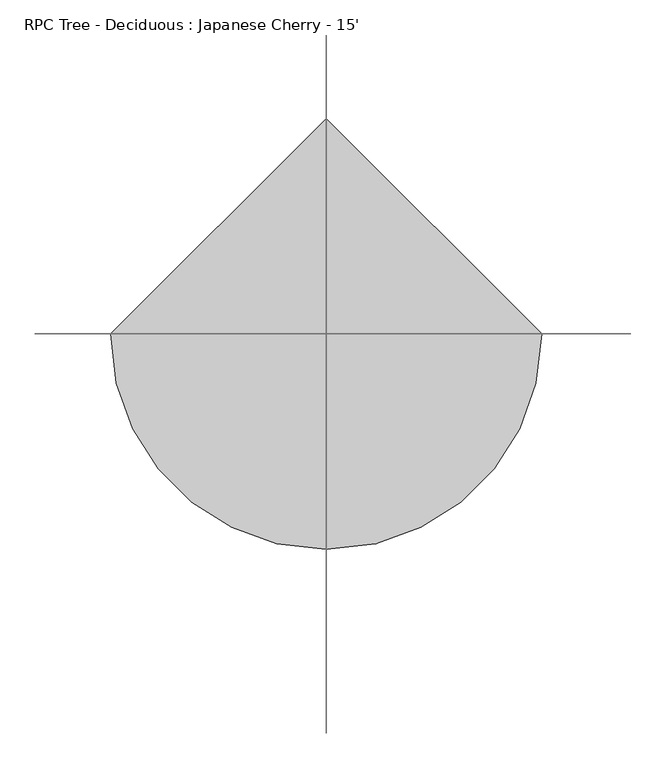
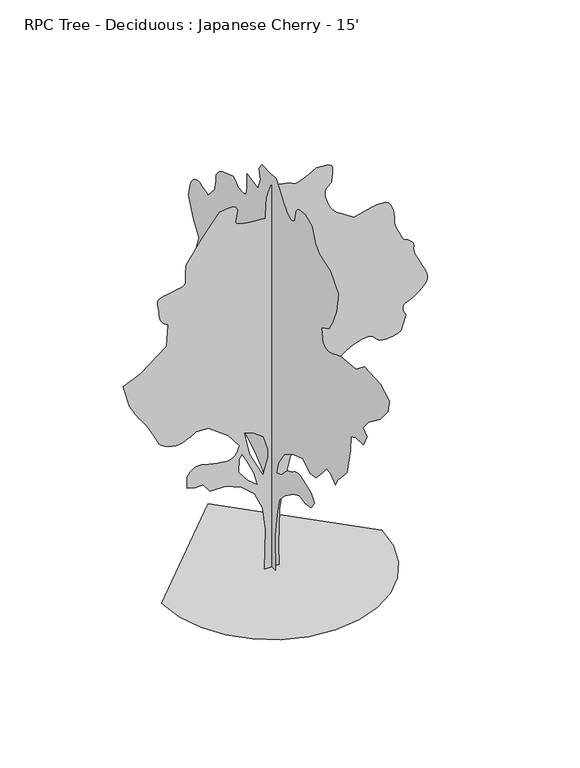
"""IFC4 building model written with IfcOpenShell, lengths in millimetres: geographic element geometry, RPC Tree - Deciduous : Japanese Cherry - 15'."""

from ifc_helpers import new_model, si_unit, origin, place, context, project, spatial, triangles, source, transform, mapped, element, save


def rpc_tree_deciduous_japanese_cherry_15_720dba75(model_context):
    return source(origin(), model_context, "Body", "Tessellation", [
        triangles([(-0.001308, 35.3573372, 0.0027784), (-0.001308, -34.1823135, 0.0027784), (-0.001308, -27.86057, 186.4945759), (-0.001308, -46.8258028, 309.7693188), (-0.001308, -68.9520821, 404.5960888), (-0.001308, -119.526734, 458.3308539), (-0.001308, -195.3869473, 512.0667818), (-0.001308, -245.9616038, 534.1922482), (-0.001308, -296.5362602, 524.7095421), (-0.001308, -350.2710254, 534.1922482), (-0.001308, -378.7190346, 575.2842167), (-0.001308, -350.2710254, 613.2148956), (-0.001308, -249.1228934, 647.984285), (-0.001308, -240.3312607, 647.275462), (-0.001308, -231.6226171, 646.3722467), (-0.001308, -223.0799154, 645.0814098), (-0.001308, -214.7861266, 643.2109571), (-0.001308, -206.8242398, 640.5664965), (-0.001308, -199.2760268, 636.9536356), (-0.001308, -192.2268386, 632.1802351), (-0.001308, -185.1764696, 627.0382524), (-0.001308, -177.6294557, 622.3929691), (-0.001308, -169.6675688, 618.1636488), (-0.001308, -161.37378, 614.2651222), (-0.001308, -152.8310783, 610.6166531), (-0.001308, -144.1224257, 607.1329631), (-0.001308, -135.3308021, 603.7322259), (-0.001308, -87.917308, 553.1575876), (-0.001308, -40.5040593, 534.1922482), (-0.001308, -59.4694078, 600.5709363), (-0.001308, -113.2044001, 679.5936201), (-0.001308, -189.0655672, 727.0070051), (-0.001308, -277.5709208, 755.4550507), (-0.001308, -340.7883556, 714.3630095), (-0.001308, -391.3629939, 720.6855886), (-0.001308, -445.0977591, 777.5804443), (-0.001308, -486.1897639, 828.1551189), (-0.001308, -524.1192438, 824.9938293), (-0.001308, -565.2112487, 787.0643131), (-0.001308, -590.4979683, 831.3164085), (-0.001308, -618.9460138, 862.9245083), (-0.001308, -669.5206884, 916.6604725), (-0.001308, -701.1287882, 1058.9006275), (-0.001308, -704.2900778, 1134.7619854), (-0.001308, -748.5433359, 1153.7261621), (-0.001308, -818.0821873, 1160.0487413), (-0.001308, -846.5301601, 1220.1000904), (-0.001308, -811.7607708, 1248.5482086), (-0.001308, -859.1741558, 1305.4441544), (-0.001308, -966.6436861, 1387.6352131), (-0.001308, -1036.1837002, 1469.8144993), (-0.001308, -1048.8264605, 1536.1932964), (-0.001308, -969.8049757, 1580.4417583), (-0.001308, -824.4035311, 1586.7714592), (-0.001308, -751.7034628, 1529.8753681), (-0.001308, -612.6245974, 1514.0631065), (-0.001308, -593.7327636, 1506.6546925), (-0.001308, -575.2842167, 1499.4952457), (-0.001308, -557.7187554, 1492.8337337), (-0.001308, -541.4820285, 1486.9188332), (-0.001308, -527.0138346, 1481.999802), (-0.001308, -514.7574969, 1478.3251717), (-0.001308, -505.1539043, 1476.1322823), (-0.001308, -496.556682, 1476.0138302), (-0.001308, -487.4604349, 1477.886681), (-0.001308, -478.5312924, 1481.0277683), (-0.001308, -470.4307331, 1484.7259438), (-0.001308, -463.8236873, 1488.2582863), (-0.001308, -459.3727598, 1490.9015842), (-0.001308, -457.7405557, 1491.9446892), (-0.001308, -441.9364695, 1567.8060471), (-0.001308, -508.3151939, 1602.5719482), (-0.001308, -539.9244927, 1653.150111), (-0.001308, -574.6939184, 1735.3293972), (-0.001308, -593.6592579, 1839.6388733), (-0.001308, -520.9591533, 1921.8180141), (-0.001308, -426.1324196, 1956.5956879), (-0.001308, -388.2017043, 1991.3615891), (-0.001308, -359.7536951, 2067.2229469), (-0.001308, -293.3749706, 2092.506142), (-0.001308, -282.5647293, 2092.4587612), (-0.001308, -271.9216108, 2092.1387226), (-0.001308, -261.6091952, 2091.2615959), (-0.001308, -251.7946416, 2089.5664959), (-0.001308, -242.6438557, 2086.7454472), (-0.001308, -234.3228157, 2082.5612549), (-0.001308, -226.9962643, 2076.705653), (-0.001308, -221.0518052, 2069.380228), (-0.001308, -216.6008778, 2061.0592243), (-0.001308, -213.3945509, 2051.9084747), (-0.001308, -211.1827128, 2042.0939575), (-0.001308, -209.7176315, 2031.7815056), (-0.001308, -208.7492131, 2021.1372425), (-0.001308, -208.0309067, 2010.3270012), (-0.001308, -202.5760071, 2004.3054211), (-0.001308, -196.8982468, 1998.7580853), (-0.001308, -190.7795614, 1994.1589474), (-0.001308, -183.9970721, 1990.9585613), (-0.001308, -176.3303344, 1989.6427986), (-0.001308, -167.5564877, 1990.674131), (-0.001308, -157.4562502, 1994.5263668), (-0.001308, -147.4484763, 2000.1212288), (-0.001308, -138.9342158, 2006.0596745), (-0.001308, -131.6633751, 2012.2709232), (-0.001308, -125.3870322, 2018.7073036), (-0.001308, -119.857446, 2025.2977444), (-0.001308, -114.8262942, 2032.0066372), (-0.001308, -110.0434738, 2038.7749741), (-0.001308, -65.7911513, 2098.8358429), (-0.001308, -37.3431262, 2133.6017441), (-0.001308, 10.0702679, 2130.436821), (-0.001308, 85.931519, 2133.6017441), (-0.001308, 114.3794283, 2095.6710651), (-0.001308, 101.7359413, 2041.9397518), (-0.001308, 123.8626885, 1981.878883), (-0.001308, 221.8495399, 2000.8442951), (-0.001308, 221.8495399, 1931.3007202), (-0.001308, 222.5773298, 1920.5378597), (-0.001308, 223.6097523, 1910.1424187), (-0.001308, 225.250259, 1900.529488), (-0.001308, 227.8034643, 1892.0898869), (-0.001308, 231.5716391, 1885.1794075), (-0.001308, 236.8617959, 1880.2128502), (-0.001308, 243.976169, 1877.5695522), (-0.001308, 252.1040159, 1876.585746), (-0.001308, 260.2318447, 1876.2655621), (-0.001308, 268.3596734, 1876.490839), (-0.001308, 276.4875203, 1877.1665245), (-0.001308, 284.6153491, 1878.1740211), (-0.001308, 292.7443769, 1879.3948769), (-0.001308, 300.8722238, 1880.73433), (-0.001308, 308.3267833, 1888.1071358), (-0.001308, 315.8097931, 1895.0769138), (-0.001308, 323.3485408, 1901.216946), (-0.001308, 330.9690422, 1906.1122868), (-0.001308, 338.700983, 1909.3482811), (-0.001308, 346.5715782, 1910.5099834), (-0.001308, 354.6069889, 1909.1823029), (-0.001308, 439.9510529, 1880.73433), (-0.001308, 452.0604155, 1872.5793045), (-0.001308, 463.6719523, 1864.2581554), (-0.001308, 474.2878015, 1855.6051952), (-0.001308, 483.4113361, 1846.4544456), (-0.001308, 490.5434953, 1836.6399284), (-0.001308, 495.1876159, 1825.9956654), (-0.001308, 496.8470713, 1814.3556782), (-0.001308, 497.2157261, 1802.4311153), (-0.001308, 498.2481485, 1791.0164051), (-0.001308, 499.8329355, 1780.0164951), (-0.001308, 501.859883, 1769.3485416), (-0.001308, 504.218678, 1758.9174923), (-0.001308, 506.7991528, 1748.6643391), (-0.001308, 509.4898679, 1738.494175), (-0.001308, 569.5472122, 1672.1155231), (-0.001308, 587.8120131, 1680.1164883), (-0.001308, 605.9393223, 1687.4063049), (-0.001308, 623.7892502, 1693.2619068), (-0.001308, 641.2243778, 1696.9600822), (-0.001308, 658.1070683, 1697.7780556), (-0.001308, 674.2987398, 1695.0043877), (-0.001308, 689.6606655, 1687.9160122), (-0.001308, 702.99568, 1676.963483), (-0.001308, 713.5108086, 1663.3439655), (-0.001308, 721.6753538, 1647.5197861), (-0.001308, 727.9599993, 1629.9294353), (-0.001308, 732.8352831, 1611.0115494), (-0.001308, 736.7705807, 1591.2046188), (-0.001308, 740.2353401, 1570.9590523), (-0.001308, 699.1433716, 1463.4967163), (-0.001308, 648.5698597, 1393.9531414), (-0.001308, 689.6606655, 1280.1609592), (-0.001308, 651.7299866, 1220.1000904), (-0.001308, 636.2483007, 1214.6475889), (-0.001308, 621.3474661, 1208.9698832), (-0.001308, 607.6070984, 1202.8535414), (-0.001308, 595.6079398, 1196.073432), (-0.001308, 585.9320769, 1188.404278), (-0.001308, 579.1590892, 1179.6316303), (-0.001308, 575.8685924, 1169.5313747), (-0.001308, 574.7911145, 1158.7863184), (-0.001308, 574.2102997, 1148.2060776), (-0.001308, 574.0443578, 1137.7656538), (-0.001308, 574.2102997, 1127.4354704), (-0.001308, 574.6251726, 1117.1870407), (-0.001308, 575.2059875, 1106.9955116), (-0.001308, 575.8685924, 1096.8301437), (-0.001308, 563.2257957, 1046.2566319), (-0.001308, 474.7204422, 1055.7393379), (-0.001308, 467.3666396, 1040.9024529), (-0.001308, 460.5936519, 1026.4520994), (-0.001308, 454.9810947, 1012.776844), (-0.001308, 451.1109821, 1000.2621283), (-0.001308, 449.5629298, 989.2965912), (-0.001308, 450.9177526, 980.2643663), (-0.001308, 455.7551027, 973.5565636), (-0.001308, 463.5972839, 967.9901882), (-0.001308, 473.2091609, 962.3136452), (-0.001308, 484.03717, 956.8030077), (-0.001308, 495.5289831, 951.7344944), (-0.001308, 507.1310366, 947.3843239), (-0.001308, 518.2909658, 944.0298775), (-0.001308, 528.4552073, 941.9472284), (-0.001308, 537.6616948, 940.1312782), (-0.001308, 546.3703566, 937.4868176), (-0.001308, 554.6641454, 934.1512653), (-0.001308, 562.626014, 930.2621859), (-0.001308, 570.3401871, 925.9582335), (-0.001308, 577.8872191, 921.3781351), (-0.001308, 585.3512621, 916.6604725), (-0.001308, 658.0525658, 954.5911514), (-0.001308, 678.9523802, 959.9263636), (-0.001308, 699.2725788, 964.7648764), (-0.001308, 718.4310751, 968.6077377), (-0.001308, 735.8483986, 970.9570856), (-0.001308, 750.9436255, 971.3162207), (-0.001308, 763.1359772, 969.1885889), (-0.001308, 771.8434399, 964.0738575), (-0.001308, 777.6042074, 956.6548336), (-0.001308, 781.5382696, 948.0754154), (-0.001308, 783.9528025, 938.5286871), (-0.001308, 785.1512032, 928.2068607), (-0.001308, 785.4368689, 917.3052732), (-0.001308, 785.1144321, 906.0162094), (-0.001308, 784.4874355, 894.5338434), (-0.001308, 773.6226191, 883.1154997), (-0.001308, 762.591897, 872.2791698), (-0.001308, 751.2292912, 862.6021442), (-0.001308, 739.3688232, 854.6675268), (-0.001308, 726.8445877, 849.0560961), (-0.001308, 713.4918417, 846.3464504), (-0.001308, 699.1433716, 847.1204584), (-0.001308, 683.9473515, 850.4560106), (-0.001308, 668.5296879, 854.4564932), (-0.001308, 653.4439808, 858.2341696), (-0.001308, 639.2436848, 860.9071169), (-0.001308, 626.4800016, 861.5886887), (-0.001308, 615.7076941, 859.3957993), (-0.001308, 607.4778912, 853.4418749), (-0.001308, 601.257268, 845.775119), (-0.001308, 596.0322962, 838.9369463), (-0.001308, 591.6359076, 832.7909552), (-0.001308, 587.9044856, 827.1974012), (-0.001308, 584.6696903, 822.0174849), (-0.001308, 581.7668152, 817.1149498), (-0.001308, 579.029882, 812.3510691), (-0.001308, 589.8021895, 810.9227406), (-0.001308, 600.1880745, 809.0522879), (-0.001308, 609.7999878, 806.2963514), (-0.001308, 618.2501987, 802.2141151), (-0.001308, 625.1523937, 796.3620741), (-0.001308, 630.1201138, 788.2982494), (-0.001308, 632.7646471, 777.5804443), (-0.001308, 633.8432877, 765.0206732), (-0.001308, 634.4240662, 751.795899), (-0.001308, 634.5900444, 738.0187603), (-0.001308, 634.4240662, 723.7994974), (-0.001308, 634.0092659, 709.2483507), (-0.001308, 633.4284147, 694.4767233), (-0.001308, 632.7646471, 679.5936201), (-0.001308, 616.5279202, 667.4937046), (-0.001308, 600.4002708, 655.9462263), (-0.001308, 584.494265, 645.5058025), (-0.001308, 568.9201429, 636.7236351), (-0.001308, 553.7893441, 630.1533239), (-0.001308, 539.2097471, 626.3472336), (-0.001308, 525.2951168, 625.8588913), (-0.001308, 511.3792874, 627.5811699), (-0.001308, 496.8008532, 629.9684515), (-0.001308, 481.6688916, 632.908025), (-0.001308, 466.0947696, 636.2897953), (-0.001308, 450.1887637, 640.0046848), (-0.001308, 434.0623135, 643.938747), (-0.001308, 417.8244238, 647.984285), (-0.001308, 322.9976538, 625.8588913), (-0.001308, 212.366852, 568.9628366), (-0.001308, 149.1494262, 534.1922482), (-0.001308, 76.4488493, 474.1360665), (-0.001308, 32.1964064, 382.4706224), (-0.001308, 19.5529194, 252.8732822), (-0.001308, 32.1964064, 123.2771319), (37.4314339, 0.0001191, 0.0), (-38.42984, 0.0001191, 0.0), (-32.1080988, 0.0001042, 214.9402233), (-47.9123962, 9.43e-05, 338.2150025), (-89.0040241, 8.93e-05, 426.719157), (-155.3831028, 8.93e-05, 486.7765014), (-237.5658772, 8.43e-05, 521.5458907), (-316.5873619, 8.43e-05, 521.5458907), (-354.5192762, 8.43e-05, 568.9592757), (-395.6100457, 8.43e-05, 568.9592757), (-436.7020506, 8.43e-05, 578.4419455), (-436.7020506, 7.94e-05, 638.4992535), (-428.5185021, 7.94e-05, 649.2348627), (-420.0030699, 7.94e-05, 659.3623695), (-410.8249964, 7.44e-05, 668.2736715), (-400.6512714, 7.44e-05, 675.3608116), (-389.1499749, 7.44e-05, 680.014452), (-375.9904221, 7.44e-05, 681.6276529), (-360.8406564, 7.44e-05, 679.5912947), (-342.8520015, 7.44e-05, 675.0383749), (-322.2094025, 7.44e-05, 669.8774254), (-300.1290097, 7.94e-05, 664.6619734), (-277.8281362, 7.94e-05, 659.943148), (-256.5217514, 7.94e-05, 656.275712), (-237.4272047, 7.94e-05, 654.2108671), (-221.7606282, 7.94e-05, 654.3033033), (-209.3205445, 7.94e-05, 657.1327091), (-198.8706373, 7.94e-05, 662.6160954), (-190.0790228, 7.44e-05, 670.3112652), (-182.6137808, 7.44e-05, 679.7750044), (-176.1454074, 7.44e-05, 690.5662788), (-170.3396572, 7.44e-05, 702.2418016), (-164.8657725, 7.44e-05, 714.360684), (-221.7606282, 6.95e-05, 790.2220419), (-326.070068, 6.45e-05, 866.0834724), (-389.2886656, 6.45e-05, 869.2435266), (-399.4896418, 6.45e-05, 863.1616304), (-409.939549, 6.45e-05, 857.1626507), (-420.8884809, 6.45e-05, 851.3295765), (-432.5818079, 6.45e-05, 845.7443069), (-445.2720217, 6.45e-05, 840.4920839), (-459.2056189, 6.45e-05, 835.6535711), (-474.6327295, 6.95e-05, 831.3128477), (-492.3807378, 6.95e-05, 829.8110498), (-512.1201216, 6.95e-05, 832.8431322), (-532.3573311, 6.45e-05, 839.5236837), (-551.6000519, 6.45e-05, 848.9696188), (-568.3535714, 6.45e-05, 860.2954536), (-581.1255389, 6.45e-05, 872.6170126), (-588.42364, 6.45e-05, 885.0488119), (-594.7924373, 6.45e-05, 900.5482292), (-604.9199441, 5.95e-05, 921.1908646), (-617.5354895, 5.95e-05, 944.764789), (-631.3682934, 5.95e-05, 969.0558208), (-645.1454321, 5.95e-05, 991.8545019), (-657.5950356, 5.46e-05, 1010.9491213), (-667.4463238, 5.46e-05, 1024.1276047), (-675.7590431, 5.46e-05, 1034.6237663), (-684.4025562, 5.46e-05, 1046.9453253), (-693.323378, 5.46e-05, 1060.7864862), (-702.4646805, 5.46e-05, 1075.8437794), (-711.7718885, 4.96e-05, 1091.8149702), (-721.1905724, 4.96e-05, 1108.3930281), (-730.6637587, 4.96e-05, 1125.2757912), (-765.4343834, 4.47e-05, 1245.3952034), (-673.7677402, 3.97e-05, 1283.3258823), (-541.011454, 3.47e-05, 1387.6352131), (-534.6888748, 2.48e-05, 1501.4154774), (-544.1075586, 2.48e-05, 1508.2548855), (-553.1386208, 2.48e-05, 1515.4143322), (-561.3956386, 2.48e-05, 1523.2375465), (-568.491063, 2.48e-05, 1532.0563396), (-574.0384352, 2.48e-05, 1542.2028133), (-577.6513324, 2.48e-05, 1554.0087788), (-578.9421693, 2.48e-05, 1567.7942745), (-580.0848321, 1.98e-05, 1583.3221058), (-582.6641078, 1.98e-05, 1599.51385), (-585.4105245, 1.98e-05, 1615.4920898), (-587.051013, 1.98e-05, 1630.3561535), (-586.3137397, 1.98e-05, 1643.2289143), (-581.9268345, 1.98e-05, 1653.2213276), (-572.6195901, 1.98e-05, 1659.4680393), (-556.3176782, 1.98e-05, 1663.3914917), (-533.9338337, 1.49e-05, 1667.2675632), (-508.6743653, 1.49e-05, 1671.4043747), (-483.7467808, 1.49e-05, 1676.1693455), (-462.357425, 1.49e-05, 1681.8589691), (-447.7138058, 1.49e-05, 1688.8287472), (-443.0234307, 1.49e-05, 1697.3987183), (-444.0096351, 1.49e-05, 1707.7111702), (-444.3320354, 1.49e-05, 1719.5169903), (-444.1009086, 1.49e-05, 1732.5675018), (-443.4288202, 1.49e-05, 1746.601965), (-442.4248481, 9.9e-06, 1761.3949574), (-441.1991961, 9.9e-06, 1776.6857391), (-439.8621411, 9.9e-06, 1792.2254883), (-360.8406564, 5e-06, 1906.0175251), (-269.1751941, -5e-06, 2019.8095619), (-249.6657745, -5e-06, 2023.0574741), (-230.9588313, -5e-06, 2025.5111034), (-213.8544611, -5e-06, 2026.3645397), (-199.156303, -5e-06, 2024.7998096), (-187.6644899, -5e-06, 2020.0348389), (-180.1814801, -5e-06, 2011.2634266), (-177.508551, 0.0, 1997.679372), (-178.8266391, 0.0, 1982.3768177), (-181.8587215, 0.0, 1968.8876701), (-185.2227058, 0.0, 1957.1290855), (-187.5353009, 0.0, 1946.9589214), (-187.4155771, 0.0, 1938.2822708), (-183.4802613, 0.0, 1930.9924541), (-174.3484423, 0.0, 1924.9829372), (-160.497816, 0.0, 1920.1111416), (-143.6601447, 0.0, 1916.2469879), (-124.3356429, 5e-06, 1913.2006622), (-103.0207194, 5e-06, 1910.830022), (-80.2125185, 5e-06, 1908.9452534), (-56.4091114, 5e-06, 1907.3924412), (-32.1080988, 5e-06, 1906.0175251), (-28.9470476, 0.0, 1991.3615891), (-28.2097697, -5e-06, 2003.4639027), (-26.1455108, -5e-06, 2015.3883202), (-22.9754531, -5e-06, 2027.1823677), (-18.9206611, -5e-06, 2038.8697357), (-14.2023194, -5e-06, 2050.4742599), (-9.0417537, -5e-06, 2062.0193401), (-3.6599567, -5e-06, 2073.5408752), (17.9133643, -5e-06, 2069.4632172), (38.8784908, -5e-06, 2065.3383236), (58.6271082, -5e-06, 2061.1066051), (76.5511414, -5e-06, 2056.6972813), (92.0422743, -5e-06, 2052.074453), (104.4923138, -5e-06, 2047.1671944), (113.2929485, -5e-06, 2041.9279793), (124.7481359, -5e-06, 2040.3988575), (143.389885, -5e-06, 2045.1757462), (165.9586564, -5e-06, 2054.0420654), (189.1912136, -5e-06, 2064.793008), (209.824311, -5e-06, 2075.2002216), (224.5959566, -9.9e-06, 2083.0709621), (230.2452666, -9.9e-06, 2086.1883591), (234.7981318, -9.9e-06, 2086.2831207), (246.5388578, -9.9e-06, 2086.1527508), (262.5918387, -9.9e-06, 2085.192635), (280.0826315, -9.9e-06, 2082.7983044), (296.1356124, -5e-06, 2078.3532269), (307.8763384, -5e-06, 2071.2530788), (312.4292218, -5e-06, 2060.8932461), (312.244313, -5e-06, 2048.8858395), (311.7286832, -5e-06, 2037.2103893), (310.9357083, -5e-06, 2025.8192242), (309.9222528, -5e-06, 2014.6415634), (308.7428189, -5e-06, 2003.6297356), (307.4520184, 0.0, 1992.7247326), (306.1066426, 0.0, 1981.878883), (298.0523014, 0.0, 1975.7151604), (290.4412652, 0.0, 1969.2077087), (283.7133147, 0.0, 1961.9652729), (278.3129358, 0.0, 1953.6560417), (274.6822526, 0.0, 1943.9125957), (273.2634075, 0.0, 1932.3675156), (274.4985247, 0.0, 1918.6532364), (277.9442991, 5e-06, 1903.4572163), (282.717627, 5e-06, 1887.9767658), (288.598082, 5e-06, 1872.7096745), (295.3616045, 5e-06, 1858.1656494), (302.7888946, 5e-06, 1844.8424801), (310.6595261, 5e-06, 1833.2261833), (318.750602, 9.9e-06, 1823.8264664), (328.2605593, 9.9e-06, 1815.2445774), (340.2596815, 9.9e-06, 1805.82117), (354.3308066, 9.9e-06, 1795.7103046), (370.0625499, 9.9e-06, 1785.0541237), (387.0365501, 9.9e-06, 1773.9712246), (404.8402599, 9.9e-06, 1762.6275856), (423.0600417, 9.9e-06, 1751.1298862), (454.760614, 9.9e-06, 1759.8065369), (485.6598907, 9.9e-06, 1767.677132), (514.95545, 9.9e-06, 1773.9357616), (541.8471225, 9.9e-06, 1777.7999153), (565.5300882, 9.9e-06, 1778.4519104), (585.2054498, 9.9e-06, 1775.0973186), (600.0695498, 9.9e-06, 1766.9303753), (610.7778351, 9.9e-06, 1753.6545868), (618.7764748, 1.49e-05, 1736.5621708), (624.4530905, 1.49e-05, 1717.2530296), (628.1951586, 1.49e-05, 1697.3394196), (630.388048, 1.49e-05, 1678.4215336), (631.4204704, 1.98e-05, 1662.0994194), (631.6788849, 1.98e-05, 1649.9853333), (634.1301161, 1.98e-05, 1637.0651917), (640.4515326, 1.98e-05, 1619.000742), (649.094973, 1.98e-05, 1598.3995285), (658.5136568, 2.48e-05, 1577.8458412), (667.15826, 2.48e-05, 1559.9473698), (673.4796764, 2.48e-05, 1547.2997406), (675.9309803, 2.48e-05, 1542.5110794), (679.2392086, 2.48e-05, 1541.1953167), (687.6894922, 2.48e-05, 1537.3904617), (699.0710649, 2.48e-05, 1531.3215008), (711.1709078, 2.48e-05, 1523.2019382), (721.7773098, 2.48e-05, 1513.2570511), (728.6795048, 2.48e-05, 1501.7118256), (729.6657091, 2.98e-05, 1488.7799114), (728.4306101, 2.98e-05, 1475.5515038), (729.8506542, 2.98e-05, 1462.7143513), (733.4813192, 2.98e-05, 1449.8771988), (738.8817163, 2.98e-05, 1436.660709), (745.608486, 2.98e-05, 1422.6618542), (753.2206667, 3.47e-05, 1407.5014423), (761.2750443, 3.47e-05, 1390.7882183), (770.4720119, 3.47e-05, 1372.6644699), (780.6647038, 3.47e-05, 1353.7585018), (790.1378901, 3.47e-05, 1334.4730511), (797.1775766, 3.97e-05, 1315.1876003), (800.0721674, 3.97e-05, 1296.2816322), (797.1041073, 3.97e-05, 1278.1577385), (786.5617275, 3.97e-05, 1261.1956924), (772.3614315, 4.47e-05, 1246.4146179), (759.2658646, 4.47e-05, 1234.2886139), (746.8340652, 4.47e-05, 1224.3672718), (734.623982, 4.47e-05, 1216.2240915), (722.1921827, 4.47e-05, 1209.4084465), (709.0977785, 4.47e-05, 1203.4699282), (694.8963198, 4.47e-05, 1197.9818184), (682.8521421, 4.47e-05, 1191.6402723), (675.9487118, 4.47e-05, 1183.6369091), (673.3315023, 4.47e-05, 1174.256159), (674.1434441, 4.96e-05, 1163.7682817), (677.5252144, 4.96e-05, 1152.451894), (682.6209789, 4.96e-05, 1140.5831417), (688.5749033, 4.96e-05, 1128.4370808), (663.2869846, 5.46e-05, 1049.4143606), (654.3945768, 5.46e-05, 1045.3877895), (644.9759657, 5.46e-05, 1041.5816992), (634.5070553, 5.46e-05, 1038.217733), (622.4628777, 5.46e-05, 1035.5175344), (608.3171205, 5.46e-05, 1033.702747), (591.5446341, 5.46e-05, 1032.9927612), (571.6215405, 5.46e-05, 1033.6103107), (553.7253582, 5.46e-05, 1037.7103512), (541.4689842, 5.46e-05, 1045.9033831), (531.9768311, 5.46e-05, 1056.0866278), (522.3744375, 5.46e-05, 1066.1583967), (509.7861797, 5.46e-05, 1074.0195448), (491.3364701, 5.46e-05, 1077.5672207), (464.1508112, 5.46e-05, 1074.7011166), (432.7181368, 5.46e-05, 1065.7720104), (403.8825059, 5.46e-05, 1053.1931997), (378.3101206, 5.46e-05, 1037.9593185), (356.6623504, 5.46e-05, 1021.0682711), (339.6053973, 5.46e-05, 1003.5122932), (327.7994682, 5.95e-05, 986.289362), (321.9118916, 5.95e-05, 970.3928759), (321.7826843, 5.95e-05, 956.2281155), (326.297634, 5.95e-05, 943.390963), (334.6838591, 5.95e-05, 931.6597023), (346.1662251, 5.95e-05, 920.8139254), (359.970615, 6.45e-05, 910.6306807), (375.3242563, 6.45e-05, 900.8896328), (391.4507066, 6.45e-05, 891.3702284), (400.859907, 6.45e-05, 885.2325216), (409.8269468, 6.45e-05, 878.8459202), (417.9085756, 6.45e-05, 871.9626921), (424.6637956, 6.45e-05, 864.3327072), (429.6493197, 6.45e-05, 855.7070709), (432.4229877, 6.45e-05, 845.8367432), (432.5427114, 6.45e-05, 834.4741373), (431.2803248, 6.95e-05, 820.6235292), (430.1838801, 6.95e-05, 803.7870569), (429.2249634, 6.95e-05, 784.4625097), (428.3774497, 6.95e-05, 763.1466597), (427.6117261, 7.44e-05, 740.3384588), (426.9028667, 7.44e-05, 716.5357693), (426.2201323, 7.44e-05, 692.2340549), (409.9466706, 7.44e-05, 680.1803576), (393.5618059, 7.44e-05, 668.956406), (376.9552614, 7.94e-05, 659.3907835), (360.0168331, 7.94e-05, 652.3131632), (342.6374797, 7.94e-05, 648.5532909), (324.7033636, 7.94e-05, 648.9396772), (306.1066426, 7.94e-05, 654.3033033), (287.4186663, 7.94e-05, 661.4176947), (269.227353, 7.94e-05, 666.7078514), (251.4496954, 7.44e-05, 670.4772434), (234.0051388, 7.44e-05, 673.0292679), (216.8094951, 7.44e-05, 674.6697201), (199.7797933, 7.44e-05, 675.7021425), (182.8318816, 7.44e-05, 676.4300051), (129.0971255, 7.94e-05, 641.6605431), (94.3275999, 8.43e-05, 562.6378956), (59.5577155, 8.93e-05, 429.8804466), (40.592485, 9.92e-05, 300.2842873), (34.2706212, 0.0001092, 110.6310379), (-44.7515835, 3.97e-05, 512.063221), (-19.4644937, 3.47e-05, 600.5685745), (-19.4644937, 2.98e-05, 644.8206699), (-41.5905346, 2.48e-05, 720.6820278), (-98.4864576, 2.48e-05, 761.774069), (-142.7391435, 2.48e-05, 777.5781189), (-114.2911161, 2.98e-05, 651.1432491), (-73.1993701, 2.98e-05, 470.9724152), (-92.1647232, 2.98e-05, 540.5112302), (-126.9350754, 2.48e-05, 616.3726244), (-152.2218132, 1.98e-05, 663.7860094), (-168.0258812, 1.98e-05, 641.6605431), (-171.1871708, 2.48e-05, 572.1205653), (-123.7737949, 2.98e-05, 512.063221), (-566.0279503, 0.0, 0.0021433), (-551.0642924, -129.6957172, 0.0021433), (-508.4467629, -248.8016739, 0.0021433), (-441.5891796, -353.9028894, 0.0021433), (-353.9028894, -441.5891796, 0.0021433), (-248.8016739, -508.4467629, 0.0021433), (-129.6957172, -551.0642924, 0.0021433), (2.47e-05, -566.0279503, 0.0021433), (129.6957172, -551.0642924, 0.0021433), (248.8016739, -508.4467629, 0.0021433), (353.9028894, -441.5891796, 0.0021433), (441.5891796, -353.9028894, 0.0021433), (508.4467629, -248.8016739, 0.0021433), (551.0642924, -129.6957172, 0.0021433), (566.0279503, 4.96e-05, 0.0021433), (-7.42e-05, 566.0279503, 0.0021433)], [[38, 39, 40], [115, 116, 117], [1, 2, 3], [280, 1, 3], [279, 280, 3], [279, 3, 4], [278, 279, 4], [278, 4, 5], [186, 187, 188], [277, 278, 5], [46, 47, 48], [45, 46, 48], [277, 5, 6], [185, 186, 188], [10, 11, 12], [9, 10, 12], [9, 12, 13], [8, 9, 13], [8, 13, 14], [8, 14, 15], [8, 15, 16], [8, 16, 17], [8, 17, 18], [8, 18, 19], [8, 19, 20], [8, 20, 21], [7, 8, 21], [7, 21, 22], [7, 22, 23], [7, 23, 24], [7, 24, 25], [7, 25, 26], [6, 7, 26], [6, 26, 27], [6, 27, 28], [277, 6, 28], [277, 28, 29], [51, 52, 53], [50, 51, 53], [50, 53, 54], [50, 54, 55], [49, 50, 55], [49, 55, 56], [48, 49, 56], [48, 56, 57], [45, 48, 57], [44, 45, 57], [44, 57, 58], [44, 58, 59], [44, 59, 60], [44, 60, 61], [44, 61, 62], [44, 62, 63], [276, 277, 29], [276, 29, 30], [184, 185, 188], [183, 184, 188], [44, 63, 64], [115, 117, 118], [111, 112, 113], [111, 113, 114], [182, 183, 188], [109, 110, 111], [109, 111, 114], [108, 109, 114], [108, 114, 115], [107, 108, 115], [106, 107, 115], [105, 106, 115], [104, 105, 115], [115, 118, 119], [170, 171, 172], [170, 172, 173], [170, 173, 174], [170, 174, 175], [74, 75, 76], [74, 76, 77], [73, 74, 77], [72, 73, 77], [71, 72, 77], [258, 259, 260], [181, 182, 188], [78, 79, 80], [170, 175, 176], [103, 104, 115], [78, 80, 81], [44, 64, 65], [275, 276, 30], [275, 30, 31], [274, 275, 31], [78, 81, 82], [78, 82, 83], [78, 83, 84], [78, 84, 85], [78, 85, 86], [78, 86, 87], [78, 87, 88], [78, 88, 89], [78, 89, 90], [78, 90, 91], [78, 91, 92], [78, 92, 93], [78, 93, 94], [78, 94, 95], [78, 95, 96], [71, 77, 78], [71, 78, 96], [71, 96, 97], [71, 97, 98], [71, 98, 99], [71, 99, 100], [115, 119, 120], [180, 181, 188], [38, 40, 41], [223, 224, 225], [33, 34, 35], [33, 35, 36], [33, 36, 37], [102, 103, 115], [179, 180, 188], [44, 65, 66], [170, 176, 177], [71, 100, 101], [43, 44, 66], [42, 43, 66], [41, 42, 66], [38, 41, 66], [37, 38, 66], [33, 37, 66], [33, 66, 67], [33, 67, 68], [33, 68, 69], [33, 69, 70], [32, 33, 70], [31, 32, 70], [274, 31, 70], [273, 274, 70], [273, 70, 71], [273, 71, 101], [273, 101, 102], [273, 102, 115], [273, 115, 120], [273, 120, 121], [273, 121, 122], [273, 122, 123], [273, 123, 124], [273, 124, 125], [273, 125, 126], [273, 126, 127], [273, 127, 128], [273, 128, 129], [273, 129, 130], [273, 130, 131], [272, 273, 131], [271, 272, 131], [270, 271, 131], [269, 270, 131], [268, 269, 131], [268, 131, 132], [268, 132, 133], [268, 133, 134], [167, 168, 169], [257, 258, 260], [257, 260, 261], [256, 257, 261], [256, 261, 262], [255, 256, 262], [255, 262, 263], [254, 255, 263], [254, 263, 264], [254, 264, 265], [254, 265, 266], [254, 266, 267], [254, 267, 268], [253, 254, 268], [252, 253, 268], [251, 252, 268], [250, 251, 268], [249, 250, 268], [248, 249, 268], [247, 248, 268], [246, 247, 268], [245, 246, 268], [166, 167, 169], [165, 166, 169], [164, 165, 169], [163, 164, 169], [162, 163, 169], [161, 162, 169], [160, 161, 169], [159, 160, 169], [158, 159, 169], [157, 158, 169], [156, 157, 169], [155, 156, 169], [154, 155, 169], [154, 169, 170], [154, 170, 177], [153, 154, 177], [153, 177, 178], [153, 178, 179], [153, 179, 188], [222, 223, 225], [222, 225, 226], [221, 222, 226], [220, 221, 226], [219, 220, 226], [218, 219, 226], [217, 218, 226], [216, 217, 226], [215, 216, 226], [214, 215, 226], [213, 214, 226], [212, 213, 226], [212, 226, 227], [212, 227, 228], [212, 228, 229], [212, 229, 230], [212, 230, 231], [211, 212, 231], [211, 231, 232], [211, 232, 233], [210, 211, 233], [209, 210, 233], [209, 233, 234], [209, 234, 235], [209, 235, 236], [209, 236, 237], [209, 237, 238], [209, 238, 239], [209, 239, 240], [208, 209, 240], [208, 240, 241], [207, 208, 241], [206, 207, 241], [206, 241, 242], [205, 206, 242], [204, 205, 242], [204, 242, 243], [203, 204, 243], [202, 203, 243], [202, 243, 244], [201, 202, 244], [201, 244, 245], [201, 245, 268], [200, 201, 268], [199, 200, 268], [198, 199, 268], [197, 198, 268], [196, 197, 268], [195, 196, 268], [194, 195, 268], [153, 188, 189], [153, 189, 190], [152, 153, 190], [152, 190, 191], [151, 152, 191], [136, 137, 138], [135, 136, 138], [135, 138, 139], [134, 135, 139], [134, 139, 140], [134, 140, 141], [134, 141, 142], [134, 142, 143], [134, 143, 144], [134, 144, 145], [134, 145, 146], [134, 146, 147], [134, 147, 148], [134, 148, 149], [134, 149, 150], [134, 150, 151], [134, 151, 191], [134, 191, 192], [134, 192, 193], [268, 134, 193], [194, 268, 193], [583, 580, 581], [574, 281, 575], [580, 583, 584], [573, 574, 575], [583, 581, 575], [580, 584, 585], [572, 573, 575], [582, 583, 575], [582, 575, 281], [571, 572, 575], [571, 575, 576], [281, 282, 283], [570, 571, 576], [570, 576, 577], [344, 345, 346], [290, 291, 292], [406, 407, 408], [570, 577, 578], [290, 292, 293], [289, 290, 293], [289, 293, 294], [289, 294, 295], [289, 295, 296], [289, 296, 297], [289, 297, 298], [289, 298, 299], [289, 299, 300], [289, 300, 301], [289, 301, 302], [289, 302, 303], [288, 289, 303], [287, 288, 303], [287, 303, 304], [287, 304, 305], [287, 305, 306], [286, 287, 306], [286, 306, 307], [286, 307, 308], [286, 308, 309], [569, 570, 578], [554, 555, 556], [405, 406, 408], [343, 344, 346], [512, 513, 514], [511, 512, 514], [511, 514, 515], [511, 515, 516], [511, 516, 517], [510, 511, 517], [510, 517, 518], [510, 518, 519], [510, 519, 520], [510, 520, 521], [510, 521, 522], [510, 522, 523], [510, 523, 524], [509, 510, 524], [509, 524, 525], [508, 509, 525], [434, 435, 436], [342, 343, 346], [507, 508, 525], [507, 525, 526], [405, 408, 409], [404, 405, 409], [403, 404, 409], [403, 409, 410], [402, 403, 410], [401, 402, 410], [400, 401, 410], [400, 410, 411], [399, 400, 411], [399, 411, 412], [399, 412, 413], [399, 413, 414], [399, 414, 415], [377, 378, 379], [341, 342, 346], [341, 346, 347], [340, 341, 347], [339, 340, 347], [338, 339, 347], [337, 338, 347], [336, 337, 347], [335, 336, 347], [334, 335, 347], [333, 334, 347], [377, 379, 380], [377, 380, 381], [377, 381, 382], [377, 382, 383], [377, 383, 384], [377, 384, 385], [377, 385, 386], [377, 386, 387], [377, 387, 388], [377, 388, 389], [377, 389, 390], [377, 390, 391], [376, 377, 391], [376, 391, 392], [375, 376, 392], [374, 375, 392], [373, 374, 392], [372, 373, 392], [372, 392, 393], [371, 372, 393], [370, 371, 393], [369, 370, 393], [369, 393, 394], [369, 394, 395], [369, 395, 396], [332, 333, 347], [369, 396, 397], [426, 427, 428], [426, 428, 429], [425, 426, 429], [425, 429, 430], [424, 425, 430], [424, 430, 431], [423, 424, 431], [423, 431, 432], [422, 423, 432], [422, 432, 433], [421, 422, 433], [420, 421, 433], [419, 420, 433], [418, 419, 433], [418, 433, 434], [418, 434, 436], [418, 436, 437], [418, 437, 438], [418, 438, 439], [417, 418, 439], [417, 439, 440], [416, 417, 440], [416, 440, 441], [415, 416, 441], [399, 415, 441], [399, 441, 442], [399, 442, 443], [399, 443, 444], [399, 444, 445], [399, 445, 446], [399, 446, 447], [399, 447, 448], [399, 448, 449], [369, 397, 398], [331, 332, 347], [368, 369, 398], [360, 361, 362], [359, 360, 362], [359, 362, 363], [358, 359, 363], [358, 363, 364], [357, 358, 364], [357, 364, 365], [356, 357, 365], [355, 356, 365], [355, 365, 366], [354, 355, 366], [353, 354, 366], [352, 353, 366], [351, 352, 366], [350, 351, 366], [349, 350, 366], [348, 349, 366], [348, 366, 367], [348, 367, 368], [348, 368, 398], [347, 348, 398], [347, 398, 399], [347, 399, 449], [347, 449, 450], [347, 450, 451], [347, 451, 452], [331, 347, 452], [331, 452, 453], [331, 453, 454], [331, 454, 455], [331, 455, 456], [330, 331, 456], [329, 330, 456], [328, 329, 456], [327, 328, 456], [326, 327, 456], [325, 326, 456], [324, 325, 456], [323, 324, 456], [322, 323, 456], [321, 322, 456], [320, 321, 456], [319, 320, 456], [318, 319, 456], [317, 318, 456], [316, 317, 456], [315, 316, 456], [314, 315, 456], [314, 456, 457], [314, 457, 458], [314, 458, 459], [314, 459, 460], [314, 460, 461], [314, 461, 462], [314, 462, 463], [314, 463, 464], [314, 464, 465], [314, 465, 466], [314, 466, 467], [314, 467, 468], [314, 468, 469], [314, 469, 470], [314, 470, 471], [314, 471, 472], [314, 472, 473], [314, 473, 474], [314, 474, 475], [314, 475, 476], [314, 476, 477], [314, 477, 478], [314, 478, 479], [314, 479, 480], [314, 480, 481], [314, 481, 482], [314, 482, 483], [314, 483, 484], [314, 484, 485], [314, 485, 486], [314, 486, 487], [314, 487, 488], [314, 488, 489], [314, 489, 490], [314, 490, 491], [314, 491, 492], [314, 492, 493], [314, 493, 494], [314, 494, 495], [314, 495, 496], [314, 496, 497], [314, 497, 498], [314, 498, 499], [314, 499, 500], [314, 500, 501], [314, 501, 502], [580, 585, 586], [554, 556, 557], [553, 554, 557], [553, 557, 558], [553, 558, 559], [553, 559, 560], [553, 560, 561], [553, 561, 562], [553, 562, 563], [552, 553, 563], [552, 563, 564], [551, 552, 564], [550, 551, 564], [550, 564, 565], [549, 550, 565], [549, 565, 566], [548, 549, 566], [547, 548, 566], [546, 547, 566], [545, 546, 566], [544, 545, 566], [543, 544, 566], [542, 543, 566], [541, 542, 566], [540, 541, 566], [539, 540, 566], [538, 539, 566], [538, 566, 567], [537, 538, 567], [537, 567, 568], [537, 568, 569], [537, 569, 578], [536, 537, 578], [535, 536, 578], [535, 578, 579], [534, 535, 579], [534, 579, 580], [533, 534, 580], [532, 533, 580], [507, 526, 527], [506, 507, 527], [531, 532, 580], [506, 527, 528], [530, 531, 580], [281, 283, 284], [582, 281, 284], [582, 284, 285], [582, 285, 286], [588, 582, 286], [587, 588, 286], [587, 286, 309], [586, 587, 309], [586, 309, 310], [586, 310, 311], [586, 311, 312], [586, 312, 313], [580, 586, 313], [580, 313, 314], [530, 580, 314], [529, 530, 314], [502, 503, 504], [502, 504, 505], [314, 502, 505], [529, 314, 505], [529, 505, 506], [529, 506, 528], [603, 604, 589], [602, 603, 589], [602, 589, 590], [601, 602, 590], [601, 590, 591], [601, 591, 592], [600, 601, 592], [599, 600, 592], [599, 592, 593], [599, 593, 594], [599, 594, 595], [599, 595, 596], [599, 596, 597], [599, 597, 598]], closed=False),
    ])


if __name__ == "__main__":
    model = new_model("IFC4")
    model_context = context("Model", 3, world=origin())
    ifc_project = project(units=[si_unit("LENGTHUNIT", "METRE", prefix="MILLI")], contexts=[model_context])
    site = spatial("IfcSite", under=ifc_project)
    building = spatial("IfcBuilding", under=site)
    placement = place(None, origin())
    rpc_tree_deciduous_japanese_cherry_15_shape = rpc_tree_deciduous_japanese_cherry_15_720dba75(model_context)
    element("IfcGeographicElement", 1, ObjectType="RPC Tree - Deciduous : Japanese Cherry - 15'", at=placement, inside=building, context=model_context, shape_type="MappedRepresentation", body=[
        mapped(rpc_tree_deciduous_japanese_cherry_15_shape, transform((0.0, 0.0, 0.0), x_axis=(1.0, 0.0, 0.0), y_axis=(0.0, 1.0, 0.0), z_axis=(0.0, 0.0, 1.0))),
    ])
    save(model, "model.ifc")

# Revit data of these elements
# Type "RPC Tree - Deciduous : Japanese Cherry - 15'"
#   built-in parameter 1005198 = "{2, 15},{39, RPC-16-FXGW-2MQ0-PN7K-A000-ST1L-LVER-AU},{1, 0},{1, 0},{2, 35},{1, 8},{5, Color},{1, 0},{1, 0},{3, 0.8},{3, 0.8},{3, 0.8},{1, 8},{7, BBoxMin},{1, 0},{1, 0},{1, 0},{1, 0},{1, 0},{1, 8},{7, BBoxMax},{1, 0},{1, 0},{1, 0},{1, 0},{1, 0},{2, 11},{9, RPCTypeId},{1, 0},{1, 0},{39, RPC-16-FXGW-2MQ0-PN7K-A000-ST1L-LVER-AU},{1, 6},{14, RPCPlantHeight},{1, 0},{1, 0},{2, 15},{2, 11},{7, keyword},{1, 0},{1, 0},{207, :Geometry:RPC:Japanese Flowering Cherry:Prunus serrulata Lindl:A landscape tree:valued for its abundant showy flowers; native to China and Japan.  Hardy only in the mildest parts of Canada and farther south.},{2, 11},{8, category},{1, 0},{1, 0},{16, :Trees [General]},{2, 11},{12, LocalizedUID},{1, 0},{1, 0},{25, Japanese Flowering Cherry},{2, 14},{6, Height},{1, 0},{1, 0},{2, 15},{1, 2},{16, Cast Reflections},{1, 0},{1, 0},{1, 0},{1, 2},{12, Cast Shadows},{1, 0},{1, 0},{1, 1},{1, 2},{9, Lock View},{1, 0},{1, 0},{1, 0},{1, 4},{5, ViewC},{1, 0},{1, 0},{1, 0},{2, 11},{20, AdvancedUIDefinition},{1, 0},{1, 0},{0, },{2, 11},{10, AssetLibID},{1, 0},{1, 0},{36, 4D3F6E72-3F99-4203-98E9-AF80B3C7A7A4},{2, 11},{10, BaseSchema},{1, 0},{1, 0},{9, RPCSchema},{2, 11},{12, ExchangeGUID},{1, 0},{1, 0},{0, },{1, 2},{6, Hidden},{1, 0},{1, 0},{1, 0},{1, 4},{11, RPCCategory},{1, 0},{1, 0},{1, 0},{2, 11},{8, RPCImage},{1, 0},{1, 0},{0, },{1, 4},{13, SchemaVersion},{1, 0},{1, 0},{1, 4},{2, 11},{12, UIDefinition},{1, 0},{1, 0},{0, },{2, 11},{6, UIName},{1, 0},{1, 0},{39, RPC-16-FXGW-2MQ0-PN7K-A000-ST1L-LVER-AU},{2, 11},{11, VersionGUID},{1, 0},{1, 0},{9, RPCSchema},{2, 11},{9, assettype},{1, 0},{1, 0},{11, RPCGeometry},{2, 11},{11, description},{1, 0},{1, 0},{0, },{2, 11},{9, localname},{1, 0},{1, 0},{3, RPC},{2, 11},{9, localtype},{1, 0},{1, 0},{3, RPC},{1, 4},{8, revision},{1, 0},{1, 0},{1, 1},{2, 11},{9, thumbnail},{1, 0},{1, 0},{0, },{1, 4},{7, version},{1, 0},{1, 0},{1, 1},{1, 2},{20, RPC_Cast Reflections},{1, 0},{1, 0},{1, 1},{1, 2},{16, RPC_Cast Shadows},{1, 0},{1, 0},{1, 1},{1, 2},{13, RPC_Lock View},{1, 0},{1, 0},{1, 0},{1, 4},{9, RPC_ViewC},{1, 0},{1, 0},{1, 0},{21, assetlibrary_base.fbx},{1, 5},"
#   built-in parameter 1005195 = "RPC-16-FXGW-2MQ0-PN7K-A000-ST1L-LVER-AU"
#   Type Comments = "Japanese Cherry"
#   Assembly Code = "G2050500"
#   Height = 7' - 0"
#   Default Elevation = 0
